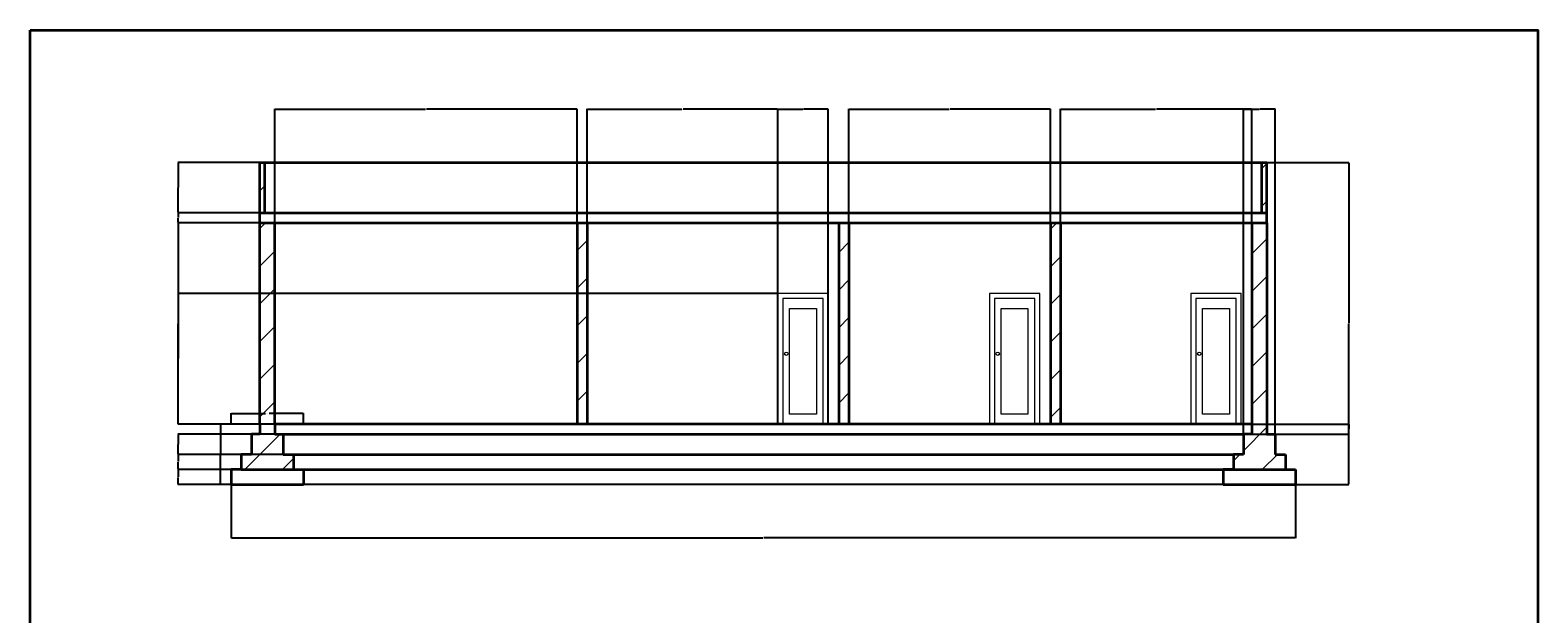
# Model space of a CAD drawing. Units: inches. Extents: x 7245 to 8143, y 15548 to 17244.
# Tile 5 of 5: x 7245 to 8143, y 16896 to 17244. Entities that reach past the tile are written whole.
import ezdxf

# ---------------------------------------------------------------- set-up
doc = ezdxf.new("R2010")
doc.units = ezdxf.units.IN
for name, color, linetype, lineweight in [('A-ANNO-DIMS', 2, 'Continuous', 18), ('A-ANNO-TTLB', 7, 'Continuous', 35), ('A-SECT', 7, 'Continuous', 35), ('A-SECT-DOOR', 3, 'Continuous', 18), ('A-SECT-PATT', 8, 'Continuous', 13), ('S-FNDN', 7, 'Continuous', 35)]:
    doc.layers.add(name, color=color, linetype=linetype, lineweight=lineweight)
doc.styles.get("Standard").update_dxf_attribs({"font": 'arial.ttf'})
doc.dimstyles.get("Standard").update_dxf_attribs({"dimtxt": 0.18, "dimasz": 0.18, "dimexe": 0.18, "dimexo": 0.0625, "dimgap": 0.09, "dimtad": 0, "dimtih": 1, "dimtoh": 1, "dimdec": 4, "dimzin": 0, "dimdsep": 46, "dimtxsty": 'Standard', "dimcen": 0.09, "dimadec": 0, "dimazin": 0, "dimtfac": 1, "dimtdec": 4, "dimtofl": 0, "dimtmove": 0, "dimatfit": 3, "dimfxl": 1, "dimtolj": 1, "dimtzin": 0, "dimarcsym": 0})

# ---------------------------------------------------------------- blocks, each defined once
blk = doc.blocks.new('*U13')
blk.add_lwpolyline([(-6.87, 0.01), (-3.87, 0.01), (-3.87, 78.01), (-33.87, 78.01), (-33.87, 0.01), (-30.87, 0.01)])
for points in [[(-30.87, 74.99), (-30.87, 0.01), (-6.87, 0.01), (-6.87, 74.99)], [(-26.87, 6.01), (-26.87, 68.99), (-10.87, 68.99), (-10.87, 6.01)]]:
    blk.add_lwpolyline(points, close=True)
blk.add_circle((-28.87, 42.01), 1)
blk = doc.blocks.new('STEPPED-FOOTING-SECTION')
for p, q in [((17, 36), (17, 30)), ((26, 36), (26, 30)), ((17, 30), (12, 30)), ((12, 30), (12, 18)), ((26, 30), (31, 30)), ((31, 30), (31, 18)), ((12, 18), (6, 18)), ((6, 18), (6, 9)), ((31, 18), (37, 18)), ((37, 18), (37, 9)), ((6, 9), (0, 9)), ((0, 9), (0, 0)), ((37, 9), (43, 9)), ((43, 9), (43, 0)), ((0, 0), (43, 0))]:
    blk.add_line(p, q)
blk = doc.blocks.new('*D38')
at = {"layer": 'A-ANNO-DIMS', "color": 0, "lineweight": -2, "transparency": 16777216}
for p, q in [((7365.08, 17009.1), (7365.08, 17015.67)), ((7365.26, 17015.49), (7385.45, 17015.49)), ((7407.9, 17015.49), (7387.71, 17015.49)), ((7408.08, 17009.1), (7408.08, 17015.67))]:
    blk.add_line(p, q, dxfattribs=at)
at = {"layer": 'A-ANNO-DIMS', "color": 0, "transparency": 16777216}
for points in [[(7365.26, 17015.52), (7365.26, 17015.46), (7365.08, 17015.49)], [(7407.9, 17015.52), (7407.9, 17015.46), (7408.08, 17015.49)]]:
    blk.add_solid(points, dxfattribs=at)
at = {"layer": 'Defpoints', "color": 0, "transparency": 16777216}
for p in [(7408.08, 17015.49), (7365.08, 17009.04), (7408.08, 17009.04)]:
    blk.add_point(p, dxfattribs=at)
at = {"layer": 'A-ANNO-DIMS', "color": 0, "transparency": 16777216, "insert": (7386.58, 17015.49), "char_height": 0.18, "attachment_point": 5}
blk.add_mtext('\\A1;FOOTING 43 TYP.', dxfattribs=at)
blk = doc.blocks.new('*D39')
at = {"layer": 'A-ANNO-DIMS', "color": 0, "lineweight": -2, "transparency": 16777216}
for p, q in [((7365.02, 17009.04), (7358.45, 17009.04)), ((7358.63, 17008.86), (7358.63, 16991.22)), ((7358.63, 16973.22), (7358.63, 16990.86)), ((7365.02, 16973.04), (7358.45, 16973.04))]:
    blk.add_line(p, q, dxfattribs=at)
at = {"layer": 'A-ANNO-DIMS', "color": 0, "transparency": 16777216}
for points in [[(7358.6, 17008.86), (7358.66, 17008.86), (7358.63, 17009.04)], [(7358.6, 16973.22), (7358.66, 16973.22), (7358.63, 16973.04)]]:
    blk.add_solid(points, dxfattribs=at)
at = {"layer": 'Defpoints', "color": 0, "transparency": 16777216}
for p in [(7358.63, 17009.04), (7365.08, 17009.04), (7365.08, 16973.04)]:
    blk.add_point(p, dxfattribs=at)
at = {"layer": 'A-ANNO-DIMS', "color": 0, "transparency": 16777216, "insert": (7358.63, 16991.04), "char_height": 0.18, "attachment_point": 5}
blk.add_mtext('\\A1;36 TYP.', dxfattribs=at)
blk = doc.blocks.new('*D53')
at = {"layer": 'A-ANNO-DIMS', "color": 0, "lineweight": -2, "transparency": 16777216}
for p, q in [((7391.08, 17009.1), (7391.08, 17196.94)), ((7391.26, 17196.76), (7480.8, 17196.76)), ((7570.9, 17196.76), (7481.36, 17196.76)), ((7571.08, 17009.1), (7571.08, 17196.94))]:
    blk.add_line(p, q, dxfattribs=at)
at = {"layer": 'A-ANNO-DIMS', "color": 0, "transparency": 16777216}
for points in [[(7391.26, 17196.79), (7391.26, 17196.73), (7391.08, 17196.76)], [(7570.9, 17196.79), (7570.9, 17196.73), (7571.08, 17196.76)]]:
    blk.add_solid(points, dxfattribs=at)
at = {"layer": 'Defpoints', "color": 0, "transparency": 16777216}
for p in [(7571.08, 17196.76), (7391.08, 17009.04), (7571.08, 17009.04)]:
    blk.add_point(p, dxfattribs=at)
at = {"layer": 'A-ANNO-DIMS', "color": 0, "transparency": 16777216, "insert": (7481.08, 17196.76), "char_height": 0.18, "attachment_point": 5}
blk.add_mtext('\\A1;180', dxfattribs=at)
blk = doc.blocks.new('*D54')
at = {"layer": 'A-ANNO-DIMS', "color": 0, "lineweight": -2, "transparency": 16777216}
for p, q in [((7577.08, 17009.1), (7577.08, 17196.94)), ((7577.26, 17196.76), (7633.46, 17196.76)), ((7690.57, 17196.76), (7634.37, 17196.76)), ((7690.75, 17009.1), (7690.75, 17196.94))]:
    blk.add_line(p, q, dxfattribs=at)
at = {"layer": 'A-ANNO-DIMS', "color": 0, "transparency": 16777216}
for points in [[(7577.26, 17196.79), (7577.26, 17196.73), (7577.08, 17196.76)], [(7690.57, 17196.79), (7690.57, 17196.73), (7690.75, 17196.76)]]:
    blk.add_solid(points, dxfattribs=at)
at = {"layer": 'Defpoints', "color": 0, "transparency": 16777216}
for p in [(7690.75, 17196.76), (7577.08, 17009.04), (7690.75, 17009.04)]:
    blk.add_point(p, dxfattribs=at)
at = {"layer": 'A-ANNO-DIMS', "color": 0, "transparency": 16777216, "insert": (7633.92, 17196.76), "char_height": 0.18, "attachment_point": 5}
blk.add_mtext('\\A1;113.67', dxfattribs=at)
blk = doc.blocks.new('*D55')
at = {"layer": 'A-ANNO-DIMS', "color": 0, "lineweight": -2, "transparency": 16777216}
for p, q in [((7690.75, 17009.1), (7690.75, 17196.94)), ((7690.93, 17196.76), (7705.53, 17196.76)), ((7720.57, 17196.76), (7705.97, 17196.76)), ((7720.75, 17009.1), (7720.75, 17196.94))]:
    blk.add_line(p, q, dxfattribs=at)
at = {"layer": 'A-ANNO-DIMS', "color": 0, "transparency": 16777216}
for points in [[(7690.93, 17196.79), (7690.93, 17196.73), (7690.75, 17196.76)], [(7720.57, 17196.79), (7720.57, 17196.73), (7720.75, 17196.76)]]:
    blk.add_solid(points, dxfattribs=at)
at = {"layer": 'Defpoints', "color": 0, "transparency": 16777216}
for p in [(7720.75, 17196.76), (7690.75, 17009.04), (7720.75, 17009.04)]:
    blk.add_point(p, dxfattribs=at)
at = {"layer": 'A-ANNO-DIMS', "color": 0, "transparency": 16777216, "insert": (7705.75, 17196.76), "char_height": 0.18, "attachment_point": 5}
blk.add_mtext('\\A1;30', dxfattribs=at)
blk = doc.blocks.new('*D56')
at = {"layer": 'A-ANNO-DIMS', "color": 0, "lineweight": -2, "transparency": 16777216}
for p, q in [((7733.08, 17009.1), (7733.08, 17196.94)), ((7733.26, 17196.76), (7792.8, 17196.76)), ((7852.9, 17196.76), (7793.36, 17196.76)), ((7853.08, 17009.1), (7853.08, 17196.94))]:
    blk.add_line(p, q, dxfattribs=at)
at = {"layer": 'A-ANNO-DIMS', "color": 0, "transparency": 16777216}
for points in [[(7733.26, 17196.79), (7733.26, 17196.73), (7733.08, 17196.76)], [(7852.9, 17196.79), (7852.9, 17196.73), (7853.08, 17196.76)]]:
    blk.add_solid(points, dxfattribs=at)
at = {"layer": 'Defpoints', "color": 0, "transparency": 16777216}
for p in [(7853.08, 17196.76), (7733.08, 17009.04), (7853.08, 17009.04)]:
    blk.add_point(p, dxfattribs=at)
at = {"layer": 'A-ANNO-DIMS', "color": 0, "transparency": 16777216, "insert": (7793.08, 17196.76), "char_height": 0.18, "attachment_point": 5}
blk.add_mtext('\\A1;120', dxfattribs=at)
blk = doc.blocks.new('*D57')
at = {"layer": 'A-ANNO-DIMS', "color": 0, "lineweight": -2, "transparency": 16777216}
for p, q in [((7859.08, 17009.1), (7859.08, 17196.94)), ((7859.26, 17196.76), (7915.8, 17196.76)), ((7972.9, 17196.76), (7916.36, 17196.76)), ((7973.08, 17009.1), (7973.08, 17196.94))]:
    blk.add_line(p, q, dxfattribs=at)
at = {"layer": 'A-ANNO-DIMS', "color": 0, "transparency": 16777216}
for points in [[(7859.26, 17196.79), (7859.26, 17196.73), (7859.08, 17196.76)], [(7972.9, 17196.79), (7972.9, 17196.73), (7973.08, 17196.76)]]:
    blk.add_solid(points, dxfattribs=at)
at = {"layer": 'Defpoints', "color": 0, "transparency": 16777216}
for p in [(7973.08, 17196.76), (7859.08, 17009.04), (7973.08, 17009.04)]:
    blk.add_point(p, dxfattribs=at)
at = {"layer": 'A-ANNO-DIMS', "color": 0, "transparency": 16777216, "insert": (7916.08, 17196.76), "char_height": 0.18, "attachment_point": 5}
blk.add_mtext('\\A1;114', dxfattribs=at)
blk = doc.blocks.new('*D58')
at = {"layer": 'A-ANNO-DIMS', "color": 0, "lineweight": -2, "transparency": 16777216}
for p, q in [((7365.083762, 16972.978782), (7365.083762, 16941.146282)), ((7999.083762, 16972.978782), (7999.083762, 16941.146282)), ((7365.263762, 16941.326282), (7681.794792, 16941.326282)), ((7998.903762, 16941.326282), (7682.372732, 16941.326282))]:
    blk.add_line(p, q, dxfattribs=at)
at = {"layer": 'A-ANNO-DIMS', "color": 0, "transparency": 16777216}
for points in [[(7365.263762, 16941.356282), (7365.263762, 16941.296282), (7365.083762, 16941.326282)], [(7998.903762, 16941.356282), (7998.903762, 16941.296282), (7999.083762, 16941.326282)]]:
    blk.add_solid(points, dxfattribs=at)
at = {"layer": 'Defpoints', "color": 0, "transparency": 16777216}
for p in [(7365.083762, 16973.041282), (7999.083762, 16973.041282), (7999.083762, 16941.326282)]:
    blk.add_point(p, dxfattribs=at)
at = {"layer": 'A-ANNO-DIMS', "color": 0, "transparency": 16777216, "insert": (7682.083762, 16941.326282), "char_height": 0.18, "attachment_point": 5}
blk.add_mtext('\\A1;634', dxfattribs=at)
blk = doc.blocks.new('*D59')
at = {"layer": 'A-ANNO-DIMS', "color": 0, "lineweight": -2, "transparency": 16777216}
for p, q in [((7982.15, 17165.04), (8030.98, 17165.04)), ((8030.8, 17164.86), (8030.8, 17069.22)), ((8030.8, 16973.22), (8030.8, 17068.86)), ((7999.15, 16973.04), (8030.98, 16973.04))]:
    blk.add_line(p, q, dxfattribs=at)
at = {"layer": 'A-ANNO-DIMS', "color": 0, "transparency": 16777216}
for points in [[(8030.77, 17164.86), (8030.83, 17164.86), (8030.8, 17165.04)], [(8030.77, 16973.22), (8030.83, 16973.22), (8030.8, 16973.04)]]:
    blk.add_solid(points, dxfattribs=at)
at = {"layer": 'Defpoints', "color": 0, "transparency": 16777216}
for p in [(7982.08, 17165.04), (8030.8, 17165.04), (7999.08, 16973.04)]:
    blk.add_point(p, dxfattribs=at)
at = {"layer": 'A-ANNO-DIMS', "color": 0, "transparency": 16777216, "insert": (8030.8, 17069.04), "char_height": 0.18, "attachment_point": 5}
blk.add_mtext('\\A1;192', dxfattribs=at)
blk = doc.blocks.new('*D60')
at = {"layer": 'A-ANNO-DIMS', "color": 0, "lineweight": -2, "transparency": 16777216}
for p, q in [((7382.02, 17165.04), (7333.19, 17165.04)), ((7333.37, 17164.86), (7333.37, 17150.22)), ((7333.37, 17135.22), (7333.37, 17149.86)), ((7382.02, 17135.04), (7333.19, 17135.04))]:
    blk.add_line(p, q, dxfattribs=at)
at = {"layer": 'A-ANNO-DIMS', "color": 0, "transparency": 16777216}
for points in [[(7333.34, 17164.86), (7333.4, 17164.86), (7333.37, 17165.04)], [(7333.34, 17135.22), (7333.4, 17135.22), (7333.37, 17135.04)]]:
    blk.add_solid(points, dxfattribs=at)
at = {"layer": 'Defpoints', "color": 0, "transparency": 16777216}
for p in [(7382.08, 17165.04), (7333.37, 17135.04), (7382.08, 17135.04)]:
    blk.add_point(p, dxfattribs=at)
at = {"layer": 'A-ANNO-DIMS', "color": 0, "transparency": 16777216, "insert": (7333.37, 17150.04), "char_height": 0.18, "attachment_point": 5}
blk.add_mtext('\\A1;30', dxfattribs=at)
blk = doc.blocks.new('*D61')
at = {"layer": 'A-ANNO-DIMS', "color": 0, "lineweight": -2, "transparency": 16777216}
for p, q in [((7382.02, 17135.04), (7333.19, 17135.04)), ((7382.02, 17129.04), (7333.19, 17129.04)), ((7333.37, 17134.86), (7333.37, 17132.22)), ((7333.37, 17129.22), (7333.37, 17131.86))]:
    blk.add_line(p, q, dxfattribs=at)
at = {"layer": 'A-ANNO-DIMS', "color": 0, "transparency": 16777216}
for points in [[(7333.34, 17134.86), (7333.4, 17134.86), (7333.37, 17135.04)], [(7333.34, 17129.22), (7333.4, 17129.22), (7333.37, 17129.04)]]:
    blk.add_solid(points, dxfattribs=at)
at = {"layer": 'Defpoints', "color": 0, "transparency": 16777216}
for p in [(7333.37, 17129.04), (7382.08, 17135.04), (7382.08, 17129.04)]:
    blk.add_point(p, dxfattribs=at)
at = {"layer": 'A-ANNO-DIMS', "color": 0, "transparency": 16777216, "insert": (7333.37, 17132.04), "char_height": 0.18, "attachment_point": 5}
blk.add_mtext('\\A1;6', dxfattribs=at)
blk = doc.blocks.new('*D62')
at = {"layer": 'A-ANNO-DIMS', "color": 0, "lineweight": -2, "transparency": 16777216}
for p, q in [((7571.02, 17129.04), (7333.19, 17129.04)), ((7333.37, 17128.86), (7333.37, 17069.22)), ((7333.37, 17009.22), (7333.37, 17068.86)), ((7571.02, 17009.04), (7333.19, 17009.04))]:
    blk.add_line(p, q, dxfattribs=at)
at = {"layer": 'A-ANNO-DIMS', "color": 0, "transparency": 16777216}
for points in [[(7333.34, 17128.86), (7333.4, 17128.86), (7333.37, 17129.04)], [(7333.34, 17009.22), (7333.4, 17009.22), (7333.37, 17009.04)]]:
    blk.add_solid(points, dxfattribs=at)
at = {"layer": 'Defpoints', "color": 0, "transparency": 16777216}
for p in [(7333.37, 17129.04), (7571.08, 17129.04), (7571.08, 17009.04)]:
    blk.add_point(p, dxfattribs=at)
at = {"layer": 'A-ANNO-DIMS', "color": 0, "transparency": 16777216, "insert": (7333.37, 17069.04), "char_height": 0.18, "attachment_point": 5}
blk.add_mtext('\\A1;120', dxfattribs=at)
blk = doc.blocks.new('*D63')
at = {"layer": 'A-ANNO-DIMS', "color": 0, "lineweight": -2, "transparency": 16777216}
for p, q in [((7690.69, 17087.04), (7333.19, 17087.04)), ((7333.37, 17086.86), (7333.37, 17048.22)), ((7333.37, 17009.22), (7333.37, 17047.86)), ((7690.69, 17009.04), (7333.19, 17009.04))]:
    blk.add_line(p, q, dxfattribs=at)
at = {"layer": 'A-ANNO-DIMS', "color": 0, "transparency": 16777216}
for points in [[(7333.34, 17086.86), (7333.4, 17086.86), (7333.37, 17087.04)], [(7333.34, 17009.22), (7333.4, 17009.22), (7333.37, 17009.04)]]:
    blk.add_solid(points, dxfattribs=at)
at = {"layer": 'Defpoints', "color": 0, "transparency": 16777216}
for p in [(7333.37, 17087.04), (7690.75, 17087.04), (7690.75, 17009.04)]:
    blk.add_point(p, dxfattribs=at)
at = {"layer": 'A-ANNO-DIMS', "color": 0, "transparency": 16777216, "insert": (7333.37, 17048.04), "char_height": 0.18, "attachment_point": 5}
blk.add_mtext('\\A1;78', dxfattribs=at)
blk = doc.blocks.new('*D64')
at = {"layer": 'A-ANNO-DIMS', "color": 0, "lineweight": -2, "transparency": 16777216}
for p, q in [((7391.15, 17009.04), (8030.98, 17009.04)), ((7391.15, 17003.04), (8030.98, 17003.04)), ((8030.8, 17008.86), (8030.8, 17006.22)), ((8030.8, 17003.22), (8030.8, 17005.86))]:
    blk.add_line(p, q, dxfattribs=at)
at = {"layer": 'A-ANNO-DIMS', "color": 0, "transparency": 16777216}
for points in [[(8030.77, 17008.86), (8030.83, 17008.86), (8030.8, 17009.04)], [(8030.77, 17003.22), (8030.83, 17003.22), (8030.8, 17003.04)]]:
    blk.add_solid(points, dxfattribs=at)
at = {"layer": 'Defpoints', "color": 0, "transparency": 16777216}
for p in [(7391.08, 17009.04), (7391.08, 17003.04), (8030.8, 17003.04)]:
    blk.add_point(p, dxfattribs=at)
at = {"layer": 'A-ANNO-DIMS', "color": 0, "transparency": 16777216, "insert": (8030.8, 17006.04), "char_height": 0.18, "attachment_point": 5}
blk.add_mtext('\\A1;6', dxfattribs=at)
blk = doc.blocks.new('*D65')
at = {"layer": 'A-ANNO-DIMS', "color": 0, "lineweight": -2, "transparency": 16777216}
for p, q in [((7956.02, 16982.04), (7333.19, 16982.04)), ((7333.37, 16981.86), (7333.37, 16977.72)), ((7333.37, 16973.22), (7333.37, 16977.36)), ((7956.02, 16973.04), (7333.19, 16973.04))]:
    blk.add_line(p, q, dxfattribs=at)
at = {"layer": 'A-ANNO-DIMS', "color": 0, "transparency": 16777216}
for points in [[(7333.34, 16981.86), (7333.4, 16981.86), (7333.37, 16982.04)], [(7333.34, 16973.22), (7333.4, 16973.22), (7333.37, 16973.04)]]:
    blk.add_solid(points, dxfattribs=at)
at = {"layer": 'Defpoints', "color": 0, "transparency": 16777216}
for p in [(7333.37, 16982.04), (7956.08, 16982.04), (7956.08, 16973.04)]:
    blk.add_point(p, dxfattribs=at)
at = {"layer": 'A-ANNO-DIMS', "color": 0, "transparency": 16777216, "insert": (7333.37, 16977.54), "char_height": 0.18, "attachment_point": 5}
blk.add_mtext('\\A1;9', dxfattribs=at)
blk = doc.blocks.new('*D66')
at = {"layer": 'A-ANNO-DIMS', "color": 0, "lineweight": -2, "transparency": 16777216}
for p, q in [((7962.02, 16991.04), (7333.19, 16991.04)), ((7333.37, 16990.86), (7333.37, 16986.72)), ((7333.37, 16982.22), (7333.37, 16986.36)), ((7962.02, 16982.04), (7333.19, 16982.04))]:
    blk.add_line(p, q, dxfattribs=at)
at = {"layer": 'A-ANNO-DIMS', "color": 0, "transparency": 16777216}
for points in [[(7333.34, 16990.86), (7333.4, 16990.86), (7333.37, 16991.04)], [(7333.34, 16982.22), (7333.4, 16982.22), (7333.37, 16982.04)]]:
    blk.add_solid(points, dxfattribs=at)
at = {"layer": 'Defpoints', "color": 0, "transparency": 16777216}
for p in [(7333.37, 16991.04), (7962.08, 16991.04), (7962.08, 16982.04)]:
    blk.add_point(p, dxfattribs=at)
at = {"layer": 'A-ANNO-DIMS', "color": 0, "transparency": 16777216, "insert": (7333.37, 16986.54), "char_height": 0.18, "attachment_point": 5}
blk.add_mtext('\\A1;9', dxfattribs=at)
blk = doc.blocks.new('*D67')
at = {"layer": 'A-ANNO-DIMS', "color": 0, "lineweight": -2, "transparency": 16777216}
for p, q in [((7968.02, 17003.04), (7333.19, 17003.04)), ((7333.37, 17002.86), (7333.37, 16997.22)), ((7333.37, 16991.22), (7333.37, 16996.86)), ((7968.02, 16991.04), (7333.19, 16991.04))]:
    blk.add_line(p, q, dxfattribs=at)
at = {"layer": 'A-ANNO-DIMS', "color": 0, "transparency": 16777216}
for points in [[(7333.34, 17002.86), (7333.4, 17002.86), (7333.37, 17003.04)], [(7333.34, 16991.22), (7333.4, 16991.22), (7333.37, 16991.04)]]:
    blk.add_solid(points, dxfattribs=at)
at = {"layer": 'Defpoints', "color": 0, "transparency": 16777216}
for p in [(7333.37, 17003.04), (7968.08, 17003.04), (7968.08, 16991.04)]:
    blk.add_point(p, dxfattribs=at)
at = {"layer": 'A-ANNO-DIMS', "color": 0, "transparency": 16777216, "insert": (7333.37, 16997.04), "char_height": 0.18, "attachment_point": 5}
blk.add_mtext('\\A1;12', dxfattribs=at)
blk = doc.blocks.new('*D68')
at = {"layer": 'A-ANNO-DIMS', "color": 0, "lineweight": -2, "transparency": 16777216}
for p, q in [((7968.08, 17003.1), (7968.08, 17196.94)), ((7968.26, 17196.76), (7977.37, 17196.76)), ((7986.9, 17196.76), (7977.79, 17196.76)), ((7987.08, 17003.1), (7987.08, 17196.94))]:
    blk.add_line(p, q, dxfattribs=at)
at = {"layer": 'A-ANNO-DIMS', "color": 0, "transparency": 16777216}
for points in [[(7968.26, 17196.79), (7968.26, 17196.73), (7968.08, 17196.76)], [(7986.9, 17196.79), (7986.9, 17196.73), (7987.08, 17196.76)]]:
    blk.add_solid(points, dxfattribs=at)
at = {"layer": 'Defpoints', "color": 0, "transparency": 16777216}
for p in [(7987.08, 17196.76), (7968.08, 17003.04), (7987.08, 17003.04)]:
    blk.add_point(p, dxfattribs=at)
at = {"layer": 'A-ANNO-DIMS', "color": 0, "transparency": 16777216, "insert": (7977.58, 17196.76), "char_height": 0.18, "attachment_point": 5}
blk.add_mtext('\\A1;19', dxfattribs=at)

msp = doc.modelspace()

# ---------------------------------------------------------------- hatches: boundary and pattern name
at = {"layer": 'A-SECT-PATT'}
h = msp.add_hatch(dxfattribs=at)
h.set_pattern_fill('ANSI31', color=256, scale=5)
h.paths.add_polyline_path([(7982.0838, 17129.0413), (7973.0838, 17129.0413), (7973.0838, 17009.0413), (7973.0838, 17003.0413), (7968.0838, 17003.0413), (7968.0838, 16991.0413), (7962.0838, 16991.0413), (7962.0838, 16982.0413), (7993.0838, 16982.0413), (7993.0838, 16991.0413), (7987.0838, 16991.0413), (7987.0838, 17003.0413), (7982.0838, 17003.0413), (7982.0838, 17009.0413)])
h.paths.add_polyline_path([(7859.0838, 17129.0413), (7853.0838, 17129.0413), (7853.0838, 17009.0413), (7859.0838, 17009.0413)])
h.paths.add_polyline_path([(7733.0838, 17129.0413), (7727.0838, 17129.0413), (7727.0838, 17009.0413), (7733.0838, 17009.0413)])
h.paths.add_polyline_path([(7577.0838, 17129.0413), (7571.0838, 17129.0413), (7571.0838, 17009.0413), (7577.0838, 17009.0413)])
h.paths.add_polyline_path([(7391.0838, 17129.0413), (7382.0838, 17129.0413), (7382.0838, 17009.0413), (7382.0838, 17003.0413), (7377.0838, 17003.0413), (7377.0838, 16991.0413), (7371.0838, 16991.0413), (7371.0838, 16982.0413), (7402.0838, 16982.0413), (7402.0838, 16991.0413), (7396.0838, 16991.0413), (7396.0838, 17003.0413), (7391.0838, 17003.0413), (7391.0838, 17009.0413)])
h.paths.add_polyline_path([(7385.0838, 17165.0413), (7382.0838, 17165.0413), (7382.0838, 17135.0413), (7385.0838, 17135.0413)])
h.paths.add_polyline_path([(7982.0838, 17165.0413), (7979.0838, 17165.0413), (7979.0838, 17135.0413), (7982.0838, 17135.0413)])

# ---------------------------------------------------------------- linework, layer by layer
at = {"layer": 'A-ANNO-TTLB'}
msp.add_lwpolyline([(7245.2864, 17243.9412), (8143.486, 17243.9412), (8143.486, 15548.1459), (7245.2864, 15548.1459)], close=True, dxfattribs=at)
at = {"layer": 'A-SECT'}
for p, q in [((7382.0838, 17165.0413), (7982.0838, 17165.0413)), ((7382.0838, 17135.0413), (7382.0838, 17165.0413)), ((7385.0838, 17135.0413), (7385.0838, 17165.0413)), ((7979.0838, 17135.0413), (7979.0838, 17165.0413)), ((7982.0838, 17135.0413), (7982.0838, 17165.0413)), ((7382.0838, 17135.0413), (7982.0838, 17135.0413)), ((7382.0838, 17129.0413), (7382.0838, 17135.0413)), ((7382.0838, 17009.0413), (7382.0838, 17129.0413)), ((7382.0838, 17129.0413), (7982.0838, 17129.0413)), ((7391.0838, 17009.0413), (7391.0838, 17129.0413)), ((7571.0838, 17129.0413), (7571.0838, 17009.0413)), ((7577.0838, 17129.0413), (7577.0838, 17009.0413)), ((7727.0838, 17129.0413), (7727.0838, 17009.0413)), ((7733.0838, 17129.0413), (7733.0838, 17009.0413)), ((7853.0838, 17129.0413), (7853.0838, 17009.0413)), ((7859.0838, 17129.0413), (7859.0838, 17009.0413)), ((7973.0838, 17129.0413), (7973.0838, 17009.0413)), ((7982.0838, 17129.0413), (7982.0838, 17135.0413)), ((7982.0838, 17129.0413), (7982.0838, 17009.0413)), ((7973.0838, 17009.0413), (7391.0838, 17009.0413))]:
    msp.add_line(p, q, dxfattribs=at)
at = {"layer": 'S-FNDN'}
for p, q in [((7396.0838, 17003.0413), (7968.0838, 17003.0413)), ((7402.0838, 16991.0413), (7962.0838, 16991.0413)), ((7371.0838, 16982.0413), (7993.0838, 16982.0413))]:
    msp.add_line(p, q, dxfattribs=at)

# ---------------------------------------------------------------- block references
at = {"layer": 'A-SECT-DOOR'}
for p in [(7724.6165, 17009.0285), (7850.6165, 17009.0285), (7970.6165, 17009.0285)]:
    msp.add_blockref('*U13', p, dxfattribs=at)
at = {"layer": 'S-FNDN'}
for p in [(7365.084, 16973.041), (7956.084, 16973.041)]:
    msp.add_blockref('STEPPED-FOOTING-SECTION', p, dxfattribs=at)

# ---------------------------------------------------------------- dimensions: what is measured, and where the dimension line sits
at = {"layer": 'A-ANNO-DIMS'}
for base, p1, p2, override, picture, middle in [((7571.0838, 17196.7563), (7391.0838, 17009.0413), (7571.0838, 17009.0413), {"dimdec": 0, "dimlfac": 1, "dimrnd": 0, "dimzin": 0, "dimdsep": 46, "dimlunit": 2}, '*D53', (7481.0838, 17196.7563)), ((7690.7498, 17196.7563), (7577.0838, 17009.0413), (7690.7498, 17009.0413), {"dimdec": 2, "dimlfac": 1, "dimrnd": 0, "dimzin": 0, "dimdsep": 46, "dimlunit": 2}, '*D54', (7633.9168, 17196.7563)), ((7720.7497, 17196.7563), (7690.7498, 17009.0413), (7720.7497, 17009.0413), {"dimdec": 0, "dimlfac": 1, "dimrnd": 0, "dimzin": 0, "dimdsep": 46, "dimlunit": 2}, '*D55', (7705.7497, 17196.7563)), ((7853.0838, 17196.7563), (7733.0838, 17009.0413), (7853.0838, 17009.0413), {"dimdec": 0, "dimlfac": 1, "dimrnd": 0, "dimzin": 0, "dimdsep": 46, "dimlunit": 2}, '*D56', (7793.0838, 17196.7563)), ((7973.0838, 17196.7563), (7859.0838, 17009.0413), (7973.0838, 17009.0413), {"dimdec": 0, "dimlfac": 1, "dimrnd": 0, "dimzin": 0, "dimdsep": 46, "dimlunit": 2}, '*D57', (7916.0838, 17196.7563)), ((7987.0838, 17196.7563), (7968.0838, 17003.0413), (7987.0838, 17003.0413), {"dimdec": 0, "dimlfac": 1, "dimrnd": 0, "dimzin": 0, "dimdsep": 46, "dimlunit": 2}, '*D68', (7977.5838, 17196.7563)), ((7999.0838, 16941.3263), (7365.0838, 16973.0413), (7999.0838, 16973.0413), {"dimdec": 0, "dimlfac": 1, "dimrnd": 0, "dimzin": 0, "dimdsep": 46, "dimlunit": 2}, '*D58', (7682.0838, 16941.3263))]:
    dim = msp.add_linear_dim(base=base, p1=p1, p2=p2, dimstyle='Standard', override=override, dxfattribs=at)
    dim.commit()
    dim.dimension.update_dxf_attribs({"geometry": picture, "text_midpoint": middle})
for base, p1, p2, picture, middle in [((7333.3688, 17135.0413), (7382.0838, 17165.0413), (7382.0838, 17135.0413), '*D60', (7333.3688, 17150.0413)), ((8030.7988, 17165.0413), (7999.0838, 16973.0413), (7982.0838, 17165.0413), '*D59', (8030.7988, 17069.0413)), ((7333.3688, 17129.0413), (7571.0838, 17009.0413), (7571.0838, 17129.0413), '*D62', (7333.3688, 17069.0413)), ((7333.3688, 17129.0413), (7382.0838, 17135.0413), (7382.0838, 17129.0413), '*D61', (7333.3688, 17132.0413)), ((7333.3688, 17087.0413), (7690.7498, 17009.0413), (7690.7498, 17087.0413), '*D63', (7333.3688, 17048.0413)), ((7333.3688, 17003.0413), (7968.0838, 16991.0413), (7968.0838, 17003.0413), '*D67', (7333.3688, 16997.0413)), ((8030.7988, 17003.0413), (7391.0838, 17009.0413), (7391.0838, 17003.0413), '*D64', (8030.7988, 17006.0413)), ((7333.3688, 16991.0413), (7962.0838, 16982.0413), (7962.0838, 16991.0413), '*D66', (7333.3688, 16986.5413)), ((7333.3688, 16982.0413), (7956.0838, 16973.0413), (7956.0838, 16982.0413), '*D65', (7333.3688, 16977.5413))]:
    dim = msp.add_linear_dim(base=base, p1=p1, p2=p2, angle=90, dimstyle='Standard', override={"dimdec": 0, "dimlfac": 1, "dimrnd": 0, "dimzin": 0, "dimdsep": 46, "dimlunit": 2}, dxfattribs=at)
    dim.commit()
    dim.dimension.update_dxf_attribs({"geometry": picture, "text_midpoint": middle})
dim = msp.add_linear_dim(base=(7408.0838, 17015.4913), p1=(7365.0838, 17009.0413), p2=(7408.0838, 17009.0413), text='FOOTING <> TYP.', dimstyle='Standard', override={"dimdec": 0, "dimlfac": 1, "dimrnd": 0, "dimzin": 0, "dimdsep": 46, "dimlunit": 2}, dxfattribs=at)
dim.commit()
dim.dimension.update_dxf_attribs({"geometry": '*D38', "text_midpoint": (7386.5838, 17015.4913)})
dim = msp.add_linear_dim(base=(7358.6338, 17009.0413), p1=(7365.0838, 16973.0413), p2=(7365.0838, 17009.0413), angle=90, text='<> TYP.', dimstyle='Standard', override={"dimdec": 0, "dimlfac": 1, "dimrnd": 0, "dimzin": 0, "dimdsep": 46, "dimlunit": 2}, dxfattribs=at)
dim.commit()
dim.dimension.update_dxf_attribs({"geometry": '*D39', "text_midpoint": (7358.6338, 16991.0413)})

doc.saveas('drawing.dxf')
